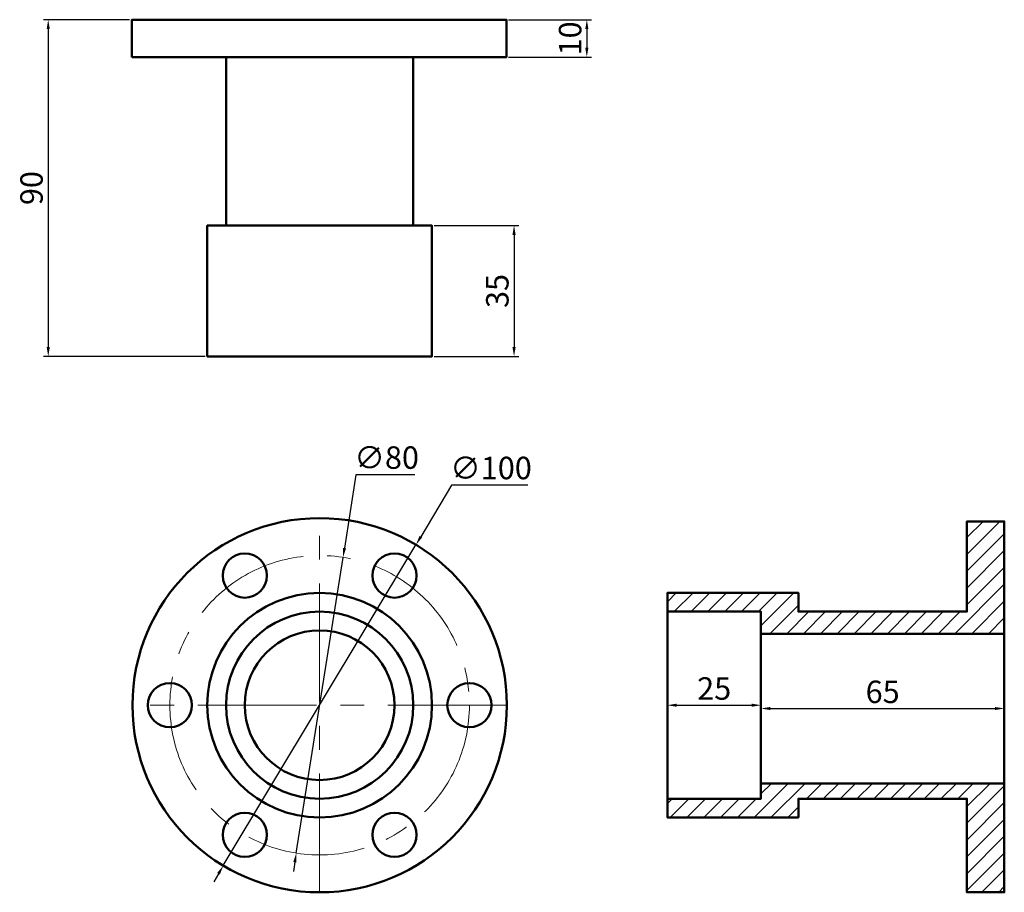
# Model space of a CAD drawing. Units: millimetres. Extents: x 133 to 396, y 57 to 290.
import ezdxf

# ---------------------------------------------------------------- set-up
doc = ezdxf.new("R2010")
doc.units = ezdxf.units.MM
doc.linetypes.add('CENTER', pattern=[50.8, 31.75, -6.35, 6.35, -6.35])
for name, color, linetype, lineweight in [('M-CNTR', 1, 'CENTER', 18), ('M-DIMS', 2, 'Continuous', 25), ('M-HATC', 8, 'Continuous', 18), ('M-OUTL', 7, 'Continuous', 50)]:
    doc.layers.add(name, color=color, linetype=linetype, lineweight=lineweight)
doc.styles.get("Standard").update_dxf_attribs({"font": 'arial.ttf'})
doc.dimstyles.new('ISO-25', dxfattribs={"dimtxt": 6, "dimasz": 2.5, "dimexe": 1.25, "dimexo": 0.625, "dimtad": 1, "dimtoh": 1, "dimdec": 0, "dimtxsty": 'Standard', "dimcen": 2.5, "dimadec": 0, "dimazin": 0, "dimtfac": 1, "dimtdec": 0, "dimtmove": 0, "dimatfit": 3, "dimfxl": 1, "dimarcsym": 0})

# ---------------------------------------------------------------- blocks, each defined once
blk = doc.blocks.new('*U1')
blk.add_circle((0, 0), 5.9)
blk = doc.blocks.new('*U2')
at = {"layer": 'M-OUTL', "color": 0, "linetype": 'ByBlock', "lineweight": -2, "transparency": 16777216}
for p, rotation in [((35.19, 141.6), 300), ((75.19, 141.6), 240), ((95.19, 106.96), 180), ((35.19, 72.32), 60.00000000000006), ((75.19, 72.32), 120)]:
    blk.add_blockref('*U1', p, dxfattribs=dict(at, rotation=rotation))
blk.add_blockref('*U1', (15.19, 106.96), dxfattribs=at)
blk = doc.blocks.new('*D3')
at = {"layer": 'Defpoints', "color": 0, "transparency": 16777216}
for p in [(242.8, 235.16), (242.8, 200.16), (264.73, 200.16)]:
    blk.add_point(p, dxfattribs=at)
at = {"layer": 'M-DIMS', "color": 0, "lineweight": -2, "transparency": 16777216}
for p, q in [((243.43, 235.16), (265.98, 235.16)), ((264.73, 232.66), (264.73, 202.66)), ((243.43, 200.16), (265.98, 200.16))]:
    blk.add_line(p, q, dxfattribs=at)
at = {"layer": 'M-DIMS', "color": 0, "transparency": 16777216}
for points in [[(264.31, 232.66), (265.15, 232.66), (264.73, 235.16)], [(264.31, 202.66), (265.15, 202.66), (264.73, 200.16)]]:
    blk.add_solid(points, dxfattribs=at)
at = {"layer": 'M-DIMS', "color": 0, "transparency": 16777216, "insert": (261.04, 217.66), "char_height": 6, "attachment_point": 5, "rotation": 90}
blk.add_mtext('35', dxfattribs=at)
blk = doc.blocks.new('*D4')
at = {"layer": 'Defpoints', "color": 0, "transparency": 16777216}
for p in [(162.67, 290.16), (140.3, 200.16), (182.8, 200.16)]:
    blk.add_point(p, dxfattribs=at)
at = {"layer": 'M-DIMS', "color": 0, "lineweight": -2, "transparency": 16777216}
for p, q in [((162.04, 290.16), (139.05, 290.16)), ((140.3, 287.66), (140.3, 202.66)), ((182.18, 200.16), (139.05, 200.16))]:
    blk.add_line(p, q, dxfattribs=at)
at = {"layer": 'M-DIMS', "color": 0, "transparency": 16777216}
for points in [[(139.89, 287.66), (140.72, 287.66), (140.3, 290.16)], [(139.89, 202.66), (140.72, 202.66), (140.3, 200.16)]]:
    blk.add_solid(points, dxfattribs=at)
at = {"layer": 'M-DIMS', "color": 0, "transparency": 16777216, "insert": (136.62, 245.16), "char_height": 6, "attachment_point": 5, "rotation": 90}
blk.add_mtext('90', dxfattribs=at)
blk = doc.blocks.new('*D5')
at = {"layer": 'Defpoints', "color": 0, "transparency": 16777216}
for p in [(262.67, 290.16), (262.67, 280.16), (284.17, 280.16)]:
    blk.add_point(p, dxfattribs=at)
at = {"layer": 'M-DIMS', "color": 0, "lineweight": -2, "transparency": 16777216}
for p, q in [((263.29, 290.16), (285.42, 290.16)), ((284.17, 287.66), (284.17, 282.66)), ((263.29, 280.16), (285.42, 280.16))]:
    blk.add_line(p, q, dxfattribs=at)
at = {"layer": 'M-DIMS', "color": 0, "transparency": 16777216}
for points in [[(283.75, 287.66), (284.59, 287.66), (284.17, 290.16)], [(283.75, 282.66), (284.59, 282.66), (284.17, 280.16)]]:
    blk.add_solid(points, dxfattribs=at)
at = {"layer": 'M-DIMS', "color": 0, "transparency": 16777216, "insert": (280.48, 285.16), "char_height": 6, "attachment_point": 5, "rotation": 90}
blk.add_mtext('10', dxfattribs=at)
blk = doc.blocks.new('*D6')
at = {"layer": 'Defpoints', "color": 0, "transparency": 16777216}
for p in [(238.53, 149.83), (187.07, 64.08)]:
    blk.add_point(p, dxfattribs=at)
at = {"layer": 'M-DIMS', "color": 0, "lineweight": -2, "transparency": 16777216}
for p, q in [((248.06, 165.73), (239.81, 151.97)), ((268.45, 165.73), (248.06, 165.73)), ((187.07, 64.08), (238.53, 149.83)), ((185.79, 61.94), (184.5, 59.8))]:
    blk.add_line(p, q, dxfattribs=at)
at = {"layer": 'M-DIMS', "color": 0, "transparency": 16777216}
for points in [[(239.46, 152.19), (240.17, 151.76), (238.53, 149.83)], [(185.43, 62.15), (186.15, 61.73), (187.07, 64.08)]]:
    blk.add_solid(points, dxfattribs=at)
at = {"layer": 'M-DIMS', "color": 0, "transparency": 16777216, "insert": (258.57, 169.58), "char_height": 6, "attachment_point": 5}
blk.add_mtext('∅100', dxfattribs=at)
blk = doc.blocks.new('*D7')
at = {"layer": 'Defpoints', "color": 0, "transparency": 16777216}
for p in [(219.04, 146.47), (206.56, 67.45)]:
    blk.add_point(p, dxfattribs=at)
at = {"layer": 'M-DIMS', "color": 0, "lineweight": -2, "transparency": 16777216}
for p, q in [((222.51, 168.5), (219.43, 148.94)), ((238.24, 168.5), (222.51, 168.5)), ((206.56, 67.45), (219.04, 146.47)), ((206.18, 64.98), (205.79, 62.51))]:
    blk.add_line(p, q, dxfattribs=at)
at = {"layer": 'M-DIMS', "color": 0, "transparency": 16777216}
for points in [[(219.01, 149), (219.84, 148.87), (219.04, 146.47)], [(205.76, 65.04), (206.59, 64.91), (206.56, 67.45)]]:
    blk.add_solid(points, dxfattribs=at)
at = {"layer": 'M-DIMS', "color": 0, "transparency": 16777216, "insert": (230.69, 172.36), "char_height": 6, "attachment_point": 5}
blk.add_mtext('∅80', dxfattribs=at)
blk = doc.blocks.new('*D8')
at = {"layer": 'Defpoints', "color": 0, "transparency": 16777216}
for p in [(330.69, 106.96), (305.69, 101.98), (330.69, 101.98)]:
    blk.add_point(p, dxfattribs=at)
at = {"layer": 'M-DIMS', "color": 0, "lineweight": -2, "transparency": 16777216}
for p, q in [((305.69, 102.61), (305.69, 108.21)), ((330.69, 102.61), (330.69, 108.21)), ((308.19, 106.96), (328.19, 106.96))]:
    blk.add_line(p, q, dxfattribs=at)
at = {"layer": 'M-DIMS', "color": 0, "transparency": 16777216}
for points in [[(308.19, 107.37), (308.19, 106.54), (305.69, 106.96)], [(328.19, 107.37), (328.19, 106.54), (330.69, 106.96)]]:
    blk.add_solid(points, dxfattribs=at)
at = {"layer": 'M-DIMS', "color": 0, "transparency": 16777216, "insert": (318.19, 110.65), "char_height": 6, "attachment_point": 5}
blk.add_mtext('25', dxfattribs=at)
blk = doc.blocks.new('*D9')
at = {"layer": 'Defpoints', "color": 0, "transparency": 16777216}
for p in [(330.69, 114.84), (395.69, 114.84), (395.69, 106.08)]:
    blk.add_point(p, dxfattribs=at)
at = {"layer": 'M-DIMS', "color": 0, "lineweight": -2, "transparency": 16777216}
for p, q in [((330.69, 114.22), (330.69, 104.83)), ((395.69, 114.22), (395.69, 104.83)), ((333.19, 106.08), (393.19, 106.08))]:
    blk.add_line(p, q, dxfattribs=at)
at = {"layer": 'M-DIMS', "color": 0, "transparency": 16777216}
for points in [[(333.19, 106.49), (333.19, 105.66), (330.69, 106.08)], [(393.19, 106.49), (393.19, 105.66), (395.69, 106.08)]]:
    blk.add_solid(points, dxfattribs=at)
at = {"layer": 'M-DIMS', "color": 0, "transparency": 16777216, "insert": (363.19, 109.76), "char_height": 6, "attachment_point": 5}
blk.add_mtext('65', dxfattribs=at)

msp = doc.modelspace()

# ---------------------------------------------------------------- hatches: boundary and pattern name
at = {"layer": 'M-HATC'}
h = msp.add_hatch(dxfattribs=at)
h.set_pattern_fill('ANSI31', color=256)
h.set_pattern_definition([(45, (157.6148, 0), (-2.245064, 2.245064), [])])
h.paths.add_polyline_path([(385.69, 131.96), (340.69, 131.96), (340.69, 136.96), (305.69, 136.96), (305.69, 131.96), (330.69, 131.96), (330.69, 126.08), (375.69, 126.08), (395.69, 126.08), (395.69, 156.08), (385.69, 156.08)])
h.paths.add_polyline_path([(395.69, 86.08), (375.69, 86.08), (330.69, 86.08), (330.69, 81.96), (305.69, 81.96), (305.69, 76.96), (340.69, 76.96), (340.69, 81.96), (385.69, 81.96), (385.69, 56.96), (395.69, 56.96)])

# ---------------------------------------------------------------- linework, layer by layer
at = {"layer": 'M-CNTR'}
for p, q in [((212.8, 56.96), (212.8, 156.96)), ((262.8, 106.96), (162.8, 106.96))]:
    msp.add_line(p, q, dxfattribs=at)
msp.add_circle((212.8, 106.96), 40, dxfattribs=at)
at = {"layer": 'M-OUTL'}
for p, q in [((187.8, 235.16), (187.8, 280.16)), ((237.8, 235.16), (237.8, 280.16)), ((305.69, 131.96), (305.69, 81.96))]:
    msp.add_line(p, q, dxfattribs=at)
for points in [[(162.67, 280.16), (162.67, 290.16), (262.67, 290.16), (262.67, 280.16)], [(182.8, 200.16), (182.8, 235.16), (242.8, 235.16), (242.8, 200.16), (212.8, 200.16)], [(395.69, 86.08), (395.69, 126.08), (395.69, 156.08), (385.69, 156.08), (385.69, 131.96), (340.69, 131.96), (340.69, 136.96), (305.69, 136.96), (305.69, 131.96), (330.69, 131.96), (330.69, 81.96), (305.69, 81.96), (305.69, 76.96), (340.69, 76.96), (340.69, 81.96), (385.69, 81.96), (385.69, 56.96), (395.69, 56.96)]]:
    msp.add_lwpolyline(points, close=True, dxfattribs=at)
for points in [[(330.69, 126.08), (375.69, 126.08), (395.69, 126.08)], [(330.69, 86.08), (375.69, 86.08), (395.69, 86.08)]]:
    msp.add_lwpolyline(points, dxfattribs=at)
for radius in [50, 30, 25, 20]:
    msp.add_circle((212.8, 106.96), radius, dxfattribs=at)

# ---------------------------------------------------------------- block references
msp.add_blockref('*U2', (157.61, 0), dxfattribs=at)

# ---------------------------------------------------------------- dimensions: what is measured, and where the dimension line sits
at = {"layer": 'M-DIMS'}
for base, p1, p2, picture, middle in [((140.3, 200.16), (162.67, 290.16), (182.8, 200.16), '*D4', (136.62, 245.16)), ((284.17, 280.16), (262.67, 290.16), (262.67, 280.16), '*D5', (280.48, 285.16)), ((264.73, 200.16), (242.8, 235.16), (242.8, 200.16), '*D3', (261.04, 217.66))]:
    dim = msp.add_linear_dim(base=base, p1=p1, p2=p2, angle=90, dimstyle='ISO-25', override={"dimclrd": 0, "dimclre": 0, "dimclrt": 0}, dxfattribs=at)
    dim.commit()
    dim.dimension.update_dxf_attribs({"geometry": picture, "text_midpoint": middle})
for p1, p2, picture, middle in [((206.56, 67.45), (219.04, 146.47), '*D7', (230.69, 168.5)), ((187.07, 64.08), (238.53, 149.83), '*D6', (258.57, 165.73))]:
    dim = msp.add_diameter_dim_2p(p1=p1, p2=p2, dimstyle='ISO-25', override={"dimclrd": 0, "dimclre": 0, "dimclrt": 0}, dxfattribs=at)
    dim.commit()
    dim.dimension.update_dxf_attribs({"geometry": picture, "text_midpoint": middle, "dimtype": 163})
for base, p1, p2, picture, middle in [((330.69, 106.96), (305.69, 101.98), (330.69, 101.98), '*D8', (318.19, 110.65)), ((395.69, 106.08), (330.69, 114.84), (395.69, 114.84), '*D9', (363.19, 109.76))]:
    dim = msp.add_linear_dim(base=base, p1=p1, p2=p2, dimstyle='ISO-25', override={"dimclrd": 0, "dimclre": 0, "dimclrt": 0}, dxfattribs=at)
    dim.commit()
    dim.dimension.update_dxf_attribs({"geometry": picture, "text_midpoint": middle})

doc.saveas('drawing.dxf')
